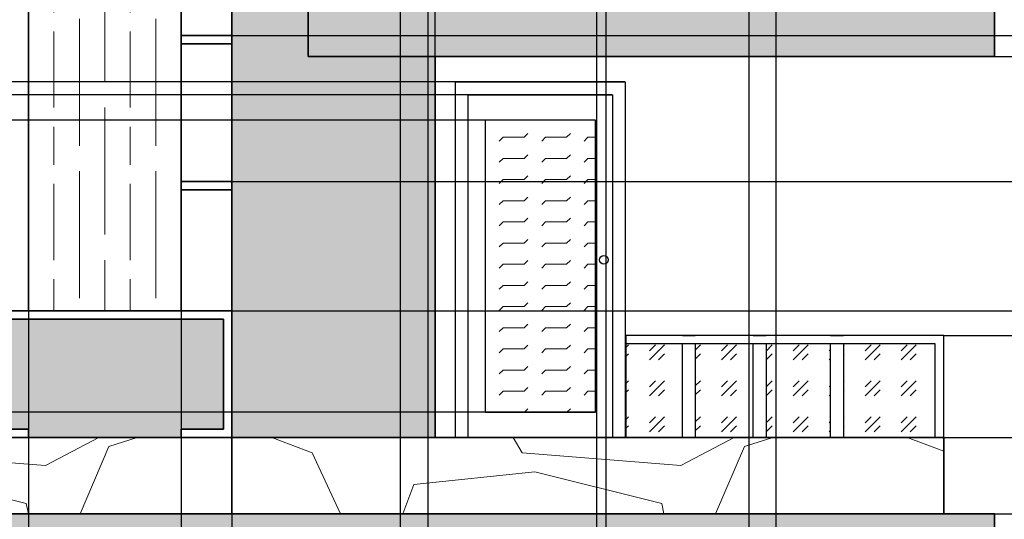
# Model space of a CAD drawing. Units: inches. Extents: x -73 to 458, y -161 to 332.
# Tile 3 of 6: x 106 to 338, y 5 to 123. Entities that reach past the tile are written whole.
import ezdxf

# ---------------------------------------------------------------- set-up
doc = ezdxf.new("R2010")
doc.units = ezdxf.units.IN
doc.header["$MEASUREMENT"] = 0
for name, color, linetype, lineweight in [('A-ANNO-DIMS', 2, 'Continuous', 18), ('A-DOOR', 4, 'Continuous', 25), ('A-ELEV', 7, 'Continuous', 35), ('A-ELEV-PATT', 8, 'Continuous', 13), ('A-GLAZ', 3, 'Continuous', 25), ('A-GLAZ-PATT', 8, 'Continuous', 13)]:
    doc.layers.add(name, color=color, linetype=linetype, lineweight=lineweight)
doc.styles.get("Standard").update_dxf_attribs({"font": 'arial.ttf'})
doc.dimstyles.get("Standard").update_dxf_attribs({"dimtxt": 12, "dimasz": 0.18, "dimexe": 0.18, "dimexo": 0.0625, "dimgap": 0.09, "dimtad": 0, "dimtih": 1, "dimtoh": 1, "dimdec": 0, "dimzin": 0, "dimdsep": 46, "dimlunit": 3, "dimtxsty": 'Standard', "dimcen": 0.09, "dimadec": 0, "dimazin": 0, "dimtfac": 1, "dimtdec": 0, "dimtofl": 0, "dimtmove": 0, "dimatfit": 3, "dimfxl": 1, "dimtolj": 1, "dimtzin": 0, "dimarcsym": 0})

# ---------------------------------------------------------------- blocks, each defined once
blk = doc.blocks.new('*U3')
blk.add_lwpolyline([(3.12, 0.01), (0.12, 0.01), (0.12, 84.01), (40.12, 84.01), (40.12, 0.01), (37.12, 0.01)])
for points in [[(37.12, 80.99), (37.12, 0.01), (3.12, 0.01), (3.12, 80.99)], [(33.12, 6.01), (33.12, 74.99), (7.12, 74.99), (7.12, 6.01)]]:
    blk.add_lwpolyline(points, close=True)
blk.add_circle((35.12, 42.01), 1)
blk = doc.blocks.new('*D7')
at = {"layer": 'A-ANNO-DIMS', "color": 0, "lineweight": -2, "transparency": 16777216}
for p, q in [((174, 126.13), (174, 324.4)), ((174.18, 324.22), (180.34, 324.22)), ((203.82, 324.22), (197.66, 324.22)), ((204, 24.13), (204, 324.4))]:
    blk.add_line(p, q, dxfattribs=at)
at = {"layer": 'A-ANNO-DIMS', "color": 0, "transparency": 16777216}
for points in [[(174.18, 324.25), (174.18, 324.19), (174, 324.22)], [(203.82, 324.25), (203.82, 324.19), (204, 324.22)]]:
    blk.add_solid(points, dxfattribs=at)
at = {"layer": 'Defpoints', "color": 0, "transparency": 16777216}
for p in [(204, 324.22), (174, 126.07), (204, 24.07)]:
    blk.add_point(p, dxfattribs=at)
at = {"layer": 'A-ANNO-DIMS', "color": 0, "transparency": 16777216, "insert": (189, 324.22), "char_height": 12, "attachment_point": 5}
blk.add_mtext('\\A1;30', dxfattribs=at)
blk = doc.blocks.new('*D8')
at = {"layer": 'A-ANNO-DIMS', "color": 0, "lineweight": -2, "transparency": 16777216}
for p, q in [((204, 24.13), (204, 324.4)), ((204.18, 324.22), (257.28, 324.22)), ((335.82, 324.22), (282.72, 324.22)), ((336, 126.13), (336, 324.4))]:
    blk.add_line(p, q, dxfattribs=at)
at = {"layer": 'A-ANNO-DIMS', "color": 0, "transparency": 16777216}
for points in [[(204.18, 324.25), (204.18, 324.19), (204, 324.22)], [(335.82, 324.25), (335.82, 324.19), (336, 324.22)]]:
    blk.add_solid(points, dxfattribs=at)
at = {"layer": 'Defpoints', "color": 0, "transparency": 16777216}
for p in [(336, 324.22), (336, 126.07), (204, 24.07)]:
    blk.add_point(p, dxfattribs=at)
at = {"layer": 'A-ANNO-DIMS', "color": 0, "transparency": 16777216, "insert": (270, 324.22), "char_height": 12, "attachment_point": 5}
blk.add_mtext('\\A1;132', dxfattribs=at)
blk = doc.blocks.new('*D18')
at = {"layer": 'A-ANNO-DIMS', "color": 0, "lineweight": -2, "transparency": 16777216}
for p, q in [((336.06, 6.07), (408.51, 6.07)), ((408.33, 6.07), (408.33, 6.25)), ((408.33, 6.25), (408.51, 6.25)), ((408.33, -5.75), (408.33, 5.89)), ((336.06, -5.93), (408.51, -5.93))]:
    blk.add_line(p, q, dxfattribs=at)
at = {"layer": 'A-ANNO-DIMS', "color": 0, "transparency": 16777216}
for points in [[(408.3, 5.89), (408.36, 5.89), (408.33, 6.07)], [(408.3, -5.75), (408.36, -5.75), (408.33, -5.93)]]:
    blk.add_solid(points, dxfattribs=at)
at = {"layer": 'Defpoints', "color": 0, "transparency": 16777216}
for p in [(336, 6.07), (408.33, 6.07), (336, -5.93)]:
    blk.add_point(p, dxfattribs=at)
at = {"layer": 'A-ANNO-DIMS', "color": 0, "transparency": 16777216, "insert": (416.56, 6.25), "char_height": 12, "attachment_point": 5}
blk.add_mtext('\\A1;12', dxfattribs=at)
blk = doc.blocks.new('*D20')
at = {"layer": 'A-ANNO-DIMS', "color": 0, "lineweight": -2, "transparency": 16777216}
for p, q in [((336.06, 114.07), (408.51, 114.07)), ((408.33, 113.89), (408.33, 66.28)), ((408.33, 6.25), (408.33, 53.85)), ((324.06, 6.07), (408.51, 6.07))]:
    blk.add_line(p, q, dxfattribs=at)
at = {"layer": 'A-ANNO-DIMS', "color": 0, "transparency": 16777216}
for points in [[(408.3, 113.89), (408.36, 113.89), (408.33, 114.07)], [(408.3, 6.25), (408.36, 6.25), (408.33, 6.07)]]:
    blk.add_solid(points, dxfattribs=at)
at = {"layer": 'Defpoints', "color": 0, "transparency": 16777216}
for p in [(336, 114.07), (408.33, 114.07), (324, 6.07)]:
    blk.add_point(p, dxfattribs=at)
at = {"layer": 'A-ANNO-DIMS', "color": 0, "transparency": 16777216, "insert": (408.33, 60.07), "char_height": 12, "attachment_point": 5}
blk.add_mtext('\\A1;108', dxfattribs=at)
blk = doc.blocks.new('*D21')
at = {"layer": 'A-ANNO-DIMS', "color": 0, "lineweight": -2, "transparency": 16777216}
for p, q in [((336.06, 126.07), (408.51, 126.07)), ((408.33, 126.07), (408.33, 126.25)), ((408.33, 126.25), (408.51, 126.25)), ((408.33, 114.25), (408.33, 125.89)), ((336.06, 114.07), (408.51, 114.07))]:
    blk.add_line(p, q, dxfattribs=at)
at = {"layer": 'A-ANNO-DIMS', "color": 0, "transparency": 16777216}
for points in [[(408.3, 125.89), (408.36, 125.89), (408.33, 126.07)], [(408.3, 114.25), (408.36, 114.25), (408.33, 114.07)]]:
    blk.add_solid(points, dxfattribs=at)
at = {"layer": 'Defpoints', "color": 0, "transparency": 16777216}
for p in [(336, 126.07), (408.33, 126.07), (336, 114.07)]:
    blk.add_point(p, dxfattribs=at)
at = {"layer": 'A-ANNO-DIMS', "color": 0, "transparency": 16777216, "insert": (416.56, 126.25), "char_height": 12, "attachment_point": 5}
blk.add_mtext('\\A1;12', dxfattribs=at)
blk = doc.blocks.new('*D36')
at = {"layer": 'A-ANNO-DIMS', "color": 0, "lineweight": -2, "transparency": 16777216}
for p, q in [((96, 53.96), (96, -153.17)), ((108, 53.96), (108, -153.17)), ((96.18, -152.99), (107.82, -152.99)), ((108, -152.99), (108.18, -152.99))]:
    blk.add_line(p, q, dxfattribs=at)
at = {"layer": 'A-ANNO-DIMS', "color": 0, "transparency": 16777216}
for points in [[(96.18, -152.96), (96.18, -153.02), (96, -152.99)], [(107.82, -152.96), (107.82, -153.02), (108, -152.99)]]:
    blk.add_solid(points, dxfattribs=at)
at = {"layer": 'Defpoints', "color": 0, "transparency": 16777216}
for p in [(96, 54.03), (108, 54.03), (108, -152.99)]:
    blk.add_point(p, dxfattribs=at)
at = {"layer": 'A-ANNO-DIMS', "color": 0, "transparency": 16777216, "insert": (116.24, -152.99), "char_height": 12, "attachment_point": 5}
blk.add_mtext('\\A1;12', dxfattribs=at)
blk = doc.blocks.new('*D37')
at = {"layer": 'A-ANNO-DIMS', "color": 0, "lineweight": -2, "transparency": 16777216}
for p, q in [((108, 53.96), (108, -153.17)), ((144, 53.96), (144, -153.17)), ((108.18, -152.99), (117.32, -152.99)), ((143.82, -152.99), (134.67, -152.99))]:
    blk.add_line(p, q, dxfattribs=at)
at = {"layer": 'A-ANNO-DIMS', "color": 0, "transparency": 16777216}
for points in [[(108.18, -152.96), (108.18, -153.02), (108, -152.99)], [(143.82, -152.96), (143.82, -153.02), (144, -152.99)]]:
    blk.add_solid(points, dxfattribs=at)
at = {"layer": 'Defpoints', "color": 0, "transparency": 16777216}
for p in [(108, 54.03), (144, 54.03), (144, -152.99)]:
    blk.add_point(p, dxfattribs=at)
at = {"layer": 'A-ANNO-DIMS', "color": 0, "transparency": 16777216, "insert": (126, -152.99), "char_height": 12, "attachment_point": 5}
blk.add_mtext('\\A1;36', dxfattribs=at)
blk = doc.blocks.new('*D38')
at = {"layer": 'A-ANNO-DIMS', "color": 0, "lineweight": -2, "transparency": 16777216}
for p, q in [((144, 53.96), (144, -153.17)), ((156, 53.96), (156, -153.17)), ((144.18, -152.99), (155.82, -152.99)), ((156, -152.99), (156.18, -152.99))]:
    blk.add_line(p, q, dxfattribs=at)
at = {"layer": 'A-ANNO-DIMS', "color": 0, "transparency": 16777216}
for points in [[(144.18, -152.96), (144.18, -153.02), (144, -152.99)], [(155.82, -152.96), (155.82, -153.02), (156, -152.99)]]:
    blk.add_solid(points, dxfattribs=at)
at = {"layer": 'Defpoints', "color": 0, "transparency": 16777216}
for p in [(144, 54.03), (156, 54.03), (156, -152.99)]:
    blk.add_point(p, dxfattribs=at)
at = {"layer": 'A-ANNO-DIMS', "color": 0, "transparency": 16777216, "insert": (164.24, -152.99), "char_height": 12, "attachment_point": 5}
blk.add_mtext('\\A1;12', dxfattribs=at)
blk = doc.blocks.new('*D39')
at = {"layer": 'A-ANNO-DIMS', "color": 0, "lineweight": -2, "transparency": 16777216}
for p, q in [((144.06, 54.03), (408.51, 54.03)), ((408.33, 53.85), (408.33, 45.26)), ((408.33, 24.25), (408.33, 32.83)), ((144.06, 24.07), (408.51, 24.07))]:
    blk.add_line(p, q, dxfattribs=at)
at = {"layer": 'A-ANNO-DIMS', "color": 0, "transparency": 16777216}
for points in [[(408.3, 53.85), (408.36, 53.85), (408.33, 54.03)], [(408.3, 24.25), (408.36, 24.25), (408.33, 24.07)]]:
    blk.add_solid(points, dxfattribs=at)
at = {"layer": 'Defpoints', "color": 0, "transparency": 16777216}
for p in [(144, 54.03), (408.33, 54.03), (144, 24.07)]:
    blk.add_point(p, dxfattribs=at)
at = {"layer": 'A-ANNO-DIMS', "color": 0, "transparency": 16777216, "insert": (408.33, 39.05), "char_height": 12, "attachment_point": 5}
blk.add_mtext('\\A1;29.96', dxfattribs=at)
blk = doc.blocks.new('*D40')
at = {"layer": 'A-ANNO-DIMS', "color": 0, "lineweight": -2, "transparency": 16777216}
for p, q in [((144.06, 84.57), (408.51, 84.57)), ((408.33, 84.39), (408.33, 75.52)), ((408.33, 54.21), (408.33, 63.08)), ((144.06, 54.03), (408.51, 54.03))]:
    blk.add_line(p, q, dxfattribs=at)
at = {"layer": 'A-ANNO-DIMS', "color": 0, "transparency": 16777216}
for points in [[(408.3, 84.39), (408.36, 84.39), (408.33, 84.57)], [(408.3, 54.21), (408.36, 54.21), (408.33, 54.03)]]:
    blk.add_solid(points, dxfattribs=at)
at = {"layer": 'Defpoints', "color": 0, "transparency": 16777216}
for p in [(144, 84.57), (408.33, 84.57), (144, 54.03)]:
    blk.add_point(p, dxfattribs=at)
at = {"layer": 'A-ANNO-DIMS', "color": 0, "transparency": 16777216, "insert": (408.33, 69.3), "char_height": 12, "attachment_point": 5}
blk.add_mtext('\\A1;30.546', dxfattribs=at)
blk = doc.blocks.new('*D41')
at = {"layer": 'A-ANNO-DIMS', "color": 0, "lineweight": -2, "transparency": 16777216}
for p, q in [((144.06, 119.06), (408.51, 119.06)), ((408.33, 118.88), (408.33, 108.04)), ((408.33, 84.75), (408.33, 95.59)), ((144.06, 84.57), (408.51, 84.57))]:
    blk.add_line(p, q, dxfattribs=at)
at = {"layer": 'A-ANNO-DIMS', "color": 0, "transparency": 16777216}
for points in [[(408.3, 118.88), (408.36, 118.88), (408.33, 119.06)], [(408.3, 84.75), (408.36, 84.75), (408.33, 84.57)]]:
    blk.add_solid(points, dxfattribs=at)
at = {"layer": 'Defpoints', "color": 0, "transparency": 16777216}
for p in [(144, 119.06), (408.33, 119.06), (144, 84.57)]:
    blk.add_point(p, dxfattribs=at)
at = {"layer": 'A-ANNO-DIMS', "color": 0, "transparency": 16777216, "insert": (408.33, 101.81), "char_height": 12, "attachment_point": 5}
blk.add_mtext('\\A1;34.484', dxfattribs=at)
blk = doc.blocks.new('*D42')
at = {"layer": 'A-ANNO-DIMS', "color": 0, "lineweight": -2, "transparency": 16777216}
for p, q in [((144.06, 149.14), (408.51, 149.14)), ((408.33, 148.96), (408.33, 140.32)), ((408.33, 119.24), (408.33, 127.88)), ((144.06, 119.06), (408.51, 119.06))]:
    blk.add_line(p, q, dxfattribs=at)
at = {"layer": 'A-ANNO-DIMS', "color": 0, "transparency": 16777216}
for points in [[(408.3, 148.96), (408.36, 148.96), (408.33, 149.14)], [(408.3, 119.24), (408.36, 119.24), (408.33, 119.06)]]:
    blk.add_solid(points, dxfattribs=at)
at = {"layer": 'Defpoints', "color": 0, "transparency": 16777216}
for p in [(144, 149.14), (408.33, 149.14), (144, 119.06)]:
    blk.add_point(p, dxfattribs=at)
at = {"layer": 'A-ANNO-DIMS', "color": 0, "transparency": 16777216, "insert": (408.33, 134.1), "char_height": 12, "attachment_point": 5}
blk.add_mtext('\\A1;30.08', dxfattribs=at)
blk = doc.blocks.new('*D65')
at = {"layer": 'A-ANNO-DIMS', "color": 0, "lineweight": -2, "transparency": 16777216}
for p, q in [((-41.6, 30.08), (-41.6, 30.26)), ((-41.6, 30.26), (-41.42, 30.26)), ((241.74, 30.08), (-41.78, 30.08)), ((-41.6, 24.26), (-41.6, 29.9)), ((248.74, 24.08), (-41.78, 24.08))]:
    blk.add_line(p, q, dxfattribs=at)
at = {"layer": 'A-ANNO-DIMS', "color": 0, "transparency": 16777216}
for points in [[(-41.63, 29.9), (-41.57, 29.9), (-41.6, 30.08)], [(-41.63, 24.26), (-41.57, 24.26), (-41.6, 24.08)]]:
    blk.add_solid(points, dxfattribs=at)
at = {"layer": 'Defpoints', "color": 0, "transparency": 16777216}
for p in [(-41.6, 30.08), (241.81, 30.08), (248.81, 24.08)]:
    blk.add_point(p, dxfattribs=at)
at = {"layer": 'A-ANNO-DIMS', "color": 0, "transparency": 16777216, "insert": (-37.37, 30.26), "char_height": 12, "attachment_point": 5}
blk.add_mtext('\\A1;6', dxfattribs=at)
blk = doc.blocks.new('*D66')
at = {"layer": 'A-ANNO-DIMS', "color": 0, "lineweight": -2, "transparency": 16777216}
for p, q in [((241.74, 99.06), (-41.78, 99.06)), ((-41.6, 98.88), (-41.6, 70.78)), ((-41.6, 30.26), (-41.6, 58.35)), ((241.74, 30.08), (-41.78, 30.08))]:
    blk.add_line(p, q, dxfattribs=at)
at = {"layer": 'A-ANNO-DIMS', "color": 0, "transparency": 16777216}
for points in [[(-41.63, 98.88), (-41.57, 98.88), (-41.6, 99.06)], [(-41.63, 30.26), (-41.57, 30.26), (-41.6, 30.08)]]:
    blk.add_solid(points, dxfattribs=at)
at = {"layer": 'Defpoints', "color": 0, "transparency": 16777216}
for p in [(-41.6, 99.06), (241.81, 99.06), (241.81, 30.08)]:
    blk.add_point(p, dxfattribs=at)
at = {"layer": 'A-ANNO-DIMS', "color": 0, "transparency": 16777216, "insert": (-41.6, 64.57), "char_height": 12, "attachment_point": 5}
blk.add_mtext('\\A1;68.98', dxfattribs=at)
blk = doc.blocks.new('*D67')
at = {"layer": 'A-ANNO-DIMS', "color": 0, "lineweight": -2, "transparency": 16777216}
for p, q in [((245.74, 105.06), (-41.78, 105.06)), ((-41.6, 105.06), (-41.6, 105.24)), ((-41.6, 105.24), (-41.42, 105.24)), ((-41.6, 99.24), (-41.6, 104.88)), ((241.74, 99.06), (-41.78, 99.06))]:
    blk.add_line(p, q, dxfattribs=at)
at = {"layer": 'A-ANNO-DIMS', "color": 0, "transparency": 16777216}
for points in [[(-41.63, 104.88), (-41.57, 104.88), (-41.6, 105.06)], [(-41.63, 99.24), (-41.57, 99.24), (-41.6, 99.06)]]:
    blk.add_solid(points, dxfattribs=at)
at = {"layer": 'Defpoints', "color": 0, "transparency": 16777216}
for p in [(-41.6, 105.06), (245.81, 105.06), (241.81, 99.06)]:
    blk.add_point(p, dxfattribs=at)
at = {"layer": 'A-ANNO-DIMS', "color": 0, "transparency": 16777216, "insert": (-37.37, 105.24), "char_height": 12, "attachment_point": 5}
blk.add_mtext('\\A1;6', dxfattribs=at)
blk = doc.blocks.new('*D68')
at = {"layer": 'A-ANNO-DIMS', "color": 0, "lineweight": -2, "transparency": 16777216}
for p, q in [((248.74, 108.08), (-41.78, 108.08)), ((-41.6, 108.08), (-41.6, 108.26)), ((-41.6, 108.26), (-41.42, 108.26)), ((-41.6, 105.24), (-41.6, 107.9)), ((245.74, 105.06), (-41.78, 105.06))]:
    blk.add_line(p, q, dxfattribs=at)
at = {"layer": 'A-ANNO-DIMS', "color": 0, "transparency": 16777216}
for points in [[(-41.63, 107.9), (-41.57, 107.9), (-41.6, 108.08)], [(-41.63, 105.24), (-41.57, 105.24), (-41.6, 105.06)]]:
    blk.add_solid(points, dxfattribs=at)
at = {"layer": 'Defpoints', "color": 0, "transparency": 16777216}
for p in [(-41.6, 108.08), (248.81, 108.08), (245.81, 105.06)]:
    blk.add_point(p, dxfattribs=at)
at = {"layer": 'A-ANNO-DIMS', "color": 0, "transparency": 16777216, "insert": (-21.09, 108.26), "char_height": 12, "attachment_point": 5}
blk.add_mtext('\\A1;3.023', dxfattribs=at)
blk = doc.blocks.new('*D70')
at = {"layer": 'A-ANNO-DIMS', "color": 0, "lineweight": -2, "transparency": 16777216}
for p, q in [((324.06, 48.19), (408.51, 48.19)), ((408.33, 48.01), (408.33, 42.35)), ((408.33, 24.25), (408.33, 29.91)), ((324.06, 24.07), (408.51, 24.07))]:
    blk.add_line(p, q, dxfattribs=at)
at = {"layer": 'A-ANNO-DIMS', "color": 0, "transparency": 16777216}
for points in [[(408.3, 48.01), (408.36, 48.01), (408.33, 48.19)], [(408.3, 24.25), (408.36, 24.25), (408.33, 24.07)]]:
    blk.add_solid(points, dxfattribs=at)
at = {"layer": 'Defpoints', "color": 0, "transparency": 16777216}
for p in [(324, 48.19), (408.33, 48.19), (324, 24.07)]:
    blk.add_point(p, dxfattribs=at)
at = {"layer": 'A-ANNO-DIMS', "color": 0, "transparency": 16777216, "insert": (408.33, 36.13), "char_height": 12, "attachment_point": 5}
blk.add_mtext('\\A1;24.125', dxfattribs=at)
blk = doc.blocks.new('*D71')
at = {"layer": 'A-ANNO-DIMS', "color": 0, "lineweight": -2, "transparency": 16777216}
for p, q in [((195.77, -5.87), (195.77, 324.4)), ((195.95, 324.22), (202.17, 324.22)), ((202.35, -5.87), (202.35, 324.4)), ((202.35, 324.22), (202.53, 324.22))]:
    blk.add_line(p, q, dxfattribs=at)
at = {"layer": 'A-ANNO-DIMS', "color": 0, "transparency": 16777216}
for points in [[(195.95, 324.25), (195.95, 324.19), (195.77, 324.22)], [(202.17, 324.25), (202.17, 324.19), (202.35, 324.22)]]:
    blk.add_solid(points, dxfattribs=at)
at = {"layer": 'Defpoints', "color": 0, "transparency": 16777216}
for p in [(202.35, 324.22), (195.77, -5.93), (202.35, -5.93)]:
    blk.add_point(p, dxfattribs=at)
at = {"layer": 'A-ANNO-DIMS', "color": 0, "transparency": 16777216, "insert": (222.95, 324.22), "char_height": 12, "attachment_point": 5}
blk.add_mtext('\\A1;6.585', dxfattribs=at)
blk = doc.blocks.new('*D72')
at = {"layer": 'A-ANNO-DIMS', "color": 0, "lineweight": -2, "transparency": 16777216}
for p, q in [((202.35, -5.87), (202.35, 324.4)), ((202.53, 324.22), (241.93, 324.22)), ((242.11, -5.87), (242.11, 324.4)), ((242.11, 324.22), (242.29, 324.22))]:
    blk.add_line(p, q, dxfattribs=at)
at = {"layer": 'A-ANNO-DIMS', "color": 0, "transparency": 16777216}
for points in [[(202.53, 324.25), (202.53, 324.19), (202.35, 324.22)], [(241.93, 324.25), (241.93, 324.19), (242.11, 324.22)]]:
    blk.add_solid(points, dxfattribs=at)
at = {"layer": 'Defpoints', "color": 0, "transparency": 16777216}
for p in [(242.11, 324.22), (202.35, -5.93), (242.11, -5.93)]:
    blk.add_point(p, dxfattribs=at)
at = {"layer": 'A-ANNO-DIMS', "color": 0, "transparency": 16777216, "insert": (262.62, 324.22), "char_height": 12, "attachment_point": 5}
blk.add_mtext('\\A1;39.76', dxfattribs=at)
blk = doc.blocks.new('*D73')
at = {"layer": 'A-ANNO-DIMS', "color": 0, "lineweight": -2, "transparency": 16777216}
for p, q in [((242.11, -5.87), (242.11, 324.4)), ((242.29, 324.22), (244.17, 324.22)), ((244.35, -5.87), (244.35, 324.4)), ((244.35, 324.22), (244.53, 324.22))]:
    blk.add_line(p, q, dxfattribs=at)
at = {"layer": 'A-ANNO-DIMS', "color": 0, "transparency": 16777216}
for points in [[(242.29, 324.25), (242.29, 324.19), (242.11, 324.22)], [(244.17, 324.25), (244.17, 324.19), (244.35, 324.22)]]:
    blk.add_solid(points, dxfattribs=at)
at = {"layer": 'Defpoints', "color": 0, "transparency": 16777216}
for p in [(244.35, 324.22), (242.11, -5.93), (244.35, -5.93)]:
    blk.add_point(p, dxfattribs=at)
at = {"layer": 'A-ANNO-DIMS', "color": 0, "transparency": 16777216, "insert": (264.95, 324.22), "char_height": 12, "attachment_point": 5}
blk.add_mtext('\\A1;2.244', dxfattribs=at)
blk = doc.blocks.new('*D74')
at = {"layer": 'A-ANNO-DIMS', "color": 0, "lineweight": -2, "transparency": 16777216}
for p, q in [((244.35, -5.87), (244.35, 324.4)), ((244.53, 324.22), (277.93, 324.22)), ((278.11, -5.87), (278.11, 324.4)), ((278.11, 324.22), (278.29, 324.22))]:
    blk.add_line(p, q, dxfattribs=at)
at = {"layer": 'A-ANNO-DIMS', "color": 0, "transparency": 16777216}
for points in [[(244.53, 324.25), (244.53, 324.19), (244.35, 324.22)], [(277.93, 324.25), (277.93, 324.19), (278.11, 324.22)]]:
    blk.add_solid(points, dxfattribs=at)
at = {"layer": 'Defpoints', "color": 0, "transparency": 16777216}
for p in [(278.11, 324.22), (244.35, -5.93), (278.11, -5.93)]:
    blk.add_point(p, dxfattribs=at)
at = {"layer": 'A-ANNO-DIMS', "color": 0, "transparency": 16777216, "insert": (303.28, 324.22), "char_height": 12, "attachment_point": 5}
blk.add_mtext('\\A1;33.756', dxfattribs=at)
blk = doc.blocks.new('*D75')
at = {"layer": 'A-ANNO-DIMS', "color": 0, "lineweight": -2, "transparency": 16777216}
for p, q in [((278.11, -5.87), (278.11, 324.4)), ((278.29, 324.22), (284.3, 324.22)), ((284.48, -5.87), (284.48, 324.4)), ((284.48, 324.22), (284.66, 324.22))]:
    blk.add_line(p, q, dxfattribs=at)
at = {"layer": 'A-ANNO-DIMS', "color": 0, "transparency": 16777216}
for points in [[(278.29, 324.25), (278.29, 324.19), (278.11, 324.22)], [(284.3, 324.25), (284.3, 324.19), (284.48, 324.22)]]:
    blk.add_solid(points, dxfattribs=at)
at = {"layer": 'Defpoints', "color": 0, "transparency": 16777216}
for p in [(284.48, 324.22), (278.11, -5.93), (284.48, -5.93)]:
    blk.add_point(p, dxfattribs=at)
at = {"layer": 'A-ANNO-DIMS', "color": 0, "transparency": 16777216, "insert": (305.03, 324.22), "char_height": 12, "attachment_point": 5}
blk.add_mtext('\\A1;6.377', dxfattribs=at)

msp = doc.modelspace()

# ---------------------------------------------------------------- hatches: boundary and pattern name
at = {"layer": 'A-ELEV-PATT'}
h = msp.add_hatch(color=256, dxfattribs=at)
h.dxf.hatch_style = 1
h.paths.add_polyline_path([(167.9979, 302.0202), (155.9979, 302.0202), (95.9979, 302.0202), (23.9979, 302.0202), (23.9979, -113.9335), (33.9979, -113.9335), (33.9979, 292.0202), (95.9979, 292.0202), (157.9979, 292.0202), (157.9979, 260.2059), (167.9979, 260.2059), (167.9979, 290.0202)])
h.paths.add_polyline_path([(335.9979, 242.2059), (323.9979, 242.2059), (95.9979, 242.2059), (95.9979, 234.0665), (95.9979, 230.2059), (323.9979, 230.2059), (335.9979, 230.2059)])
h.paths.add_polyline_path([(335.9979, 126.0665), (323.9979, 126.0665), (173.9979, 126.0665), (173.9979, 114.0665), (323.9979, 114.0665), (335.9979, 114.0665)])
h.paths.add_polyline_path([(335.9979, 6.0665), (323.9979, 6.0665), (95.9979, 6.0665), (95.9979, -5.9335), (323.9979, -5.9335), (335.9979, -5.9335)])
h = msp.add_hatch(dxfattribs=at)
h.set_pattern_fill('GRAVEL', color=256, scale=150)
h.paths.add_polyline_path([(95.9979, 234.0665), (95.9979, 260.2059), (155.9979, 260.2059), (155.9979, 290.0202), (95.9979, 290.0202), (55.9979, 290.0202), (55.9979, -113.9335), (95.9979, -113.9335), (95.9979, 24.0665), (95.9979, 54.0267)])
h.paths.add_polyline_path([(323.9979, 144.0665), (248.9979, 144.0665), (173.9979, 144.0665), (173.9979, 126.0665), (323.9979, 126.0665)])
h.paths.add_polyline_path([(323.9979, 24.0665), (248.9979, 24.0665), (155.9979, 24.0665), (155.9979, 6.0665), (323.9979, 6.0665)])
h.paths.add_polyline_path([(323.9979, 260.2059), (95.9979, 260.2059), (95.9979, 242.2059), (323.9979, 242.2059)])
h.paths.add_polyline_path([(155.9979, 24.0665), (95.9979, 24.0665), (95.9979, 6.0665), (155.9979, 6.0665)], flags=17)
h = msp.add_hatch(color=256, dxfattribs=at)
h.dxf.hatch_style = 1
h.paths.add_polyline_path([(195.7666, -5.9335), (155.3839, -5.9335), (155.3839, -113.9335), (195.7666, -113.9335)])
h.paths.add_polyline_path([(323.9979, -5.9335), (284.4845, -5.9335), (284.4845, -113.9335), (323.9979, -113.9335)])
h.paths.add_polyline_path([(203.9979, 114.0665), (173.9979, 114.0665), (173.9979, 144.0665), (203.9979, 144.0665), (203.9979, 230.2059), (155.9979, 230.2059), (155.9979, 24.0665), (203.9979, 24.0665)])
h = msp.add_hatch(dxfattribs=at)
h.set_pattern_fill('FLEX', color=256, scale=20)
h.paths.add_polyline_path([(241.805, 219.0563), (215.805, 219.0563), (215.805, 150.0793), (241.805, 150.0793)])
h.paths.add_polyline_path([(241.805, 99.0563), (215.805, 99.0563), (215.805, 30.0793), (241.805, 30.0793)])
h.paths.add_polyline_path([(138.915, -38.9437), (112.915, -38.9437), (112.915, -107.9207), (138.915, -107.9207)])
h = msp.add_hatch(dxfattribs=at)
h.set_pattern_fill('GOST_WOOD', color=256, scale=3)
h.set_pattern_definition([(90, (0, 0), (18, -1e-15), [30, -6]), (90, (6, -6), (18, -1e-15), [18, -4.5, 9, -4.5]), (90, (12, -15), (18, -1e-15), [30, -6])])
h.paths.add_polyline_path([(143.9979, 215.8003), (107.9979, 215.8003), (107.9979, 54.0267), (143.9979, 54.0267)])
h = msp.add_hatch(color=256, dxfattribs=at)
h.dxf.hatch_style = 1
h.paths.add_polyline_path([(153.9979, 52.0267), (97.9979, 52.0267), (97.9979, 26.0665), (107.9979, 26.0665), (107.9979, 24.0665), (143.9979, 24.0665), (143.9979, 26.0665), (153.9979, 26.0665)])

# ---------------------------------------------------------------- linework, layer by layer
at = {"layer": 'A-ELEV'}
for p, q in [((155.9979, 6.0665), (155.9979, 230.2059)), ((107.9979, 215.8003), (107.9979, 54.0267)), ((143.9979, 54.0267), (143.9979, 215.8003)), ((173.9979, 144.0665), (173.9979, 114.0665)), ((323.9979, 114.0665), (173.9979, 114.0665)), ((203.9979, 24.0665), (203.9979, 114.0665)), ((107.9979, 26.0665), (107.9979, 24.0665)), ((143.9979, 24.0665), (143.9979, 26.0665)), ((95.9979, 24.0665), (143.9979, 24.0665)), ((155.9979, 24.0665), (323.9979, 24.0665)), ((323.9979, 6.0665), (323.9979, 24.0665)), ((95.9979, 6.0665), (323.9979, 6.0665))]:
    msp.add_line(p, q, dxfattribs=at)
for points in [[(323.9979, 126.0665), (335.9979, 126.0665), (335.9979, 114.0665), (323.9979, 114.0665)], [(155.9979, 56.0043), (155.9979, 54.0267), (143.9979, 54.0267), (143.9979, 56.0043)], [(143.9979, 26.0665), (153.9979, 26.0665), (153.9979, 52.0267), (97.9979, 52.0267), (97.9979, 26.0665), (107.9979, 26.0665)], [(143.9979, 24.6791), (143.9979, 25.9247)], [(155.9979, 25.9247), (155.9979, 24.6791)], [(323.9979, 6.0665), (335.9979, 6.0665), (335.9979, -5.9335), (323.9979, -5.9335)]]:
    msp.add_lwpolyline(points, dxfattribs=at)
for points in [[(143.9979, 119.0564), (155.9979, 119.0564), (155.9979, 117.0789), (143.9979, 117.0789)], [(143.9979, 84.5727), (155.9979, 84.5727), (155.9979, 82.5952), (143.9979, 82.5952)], [(95.9979, 24.0665), (155.9979, 24.0665), (155.9979, 54.0267), (95.9979, 54.0267)]]:
    msp.add_lwpolyline(points, close=True, dxfattribs=at)
at = {"layer": 'A-GLAZ'}
for p, q in [((248.9979, 48.1912), (248.9979, 24.0665)), ((248.9979, 24.0665), (323.9979, 24.0665))]:
    msp.add_line(p, q, dxfattribs=at)
for points in [[(323.9979, 24.0665), (323.9979, 48.1912), (248.9979, 48.1912)], [(262.3267, 48.1912), (265.3698, 48.1912)], [(279.0639, 48.1912), (282.107, 48.1912)], [(297.3226, 48.1912), (300.3657, 48.1912)], [(321.9979, 24.0665), (321.9979, 46.1912), (248.9979, 46.1912)], [(265.3698, 46.1912), (265.3698, 24.0665), (262.3267, 24.0665), (262.3267, 46.1912)], [(282.107, 46.1912), (282.107, 24.0665), (279.0639, 24.0665), (279.0639, 46.1912)], [(300.3657, 46.1912), (300.3657, 24.0665), (297.3226, 24.0665), (297.3226, 46.1912)]]:
    msp.add_lwpolyline(points, dxfattribs=at)
at = {"layer": 'A-GLAZ-PATT'}
for p, q in [((248.9979, 45.3511), (249.6087, 45.9619)), ((254.5584, 42.4264), (258.094, 45.9619)), ((254.5584, 44.5477), (255.9727, 45.9619)), ((265.3698, 44.7525), (266.5793, 45.9619)), ((271.529, 42.4264), (275.0645, 45.9619)), ((271.529, 44.5477), (272.9432, 45.9619)), ((282.107, 44.5191), (283.5498, 45.9619)), ((288.4996, 42.4264), (292.0351, 45.9619)), ((288.4996, 44.5477), (289.9138, 45.9619)), ((296.9848, 44.5477), (297.3226, 44.8855)), ((300.3657, 45.8073), (300.5204, 45.9619)), ((305.4701, 42.4264), (309.0057, 45.9619)), ((305.4701, 44.5477), (306.8843, 45.9619)), ((313.9554, 42.4264), (317.4909, 45.9619)), ((313.9554, 44.5477), (315.3696, 45.9619)), ((248.9979, 43.2298), (249.6087, 43.8406)), ((256.6798, 42.4264), (258.094, 43.8406)), ((265.3698, 42.6312), (266.5793, 43.8406)), ((273.6503, 42.4264), (275.0645, 43.8406)), ((282.1356, 42.4264), (283.5498, 43.8406)), ((290.6209, 42.4264), (292.0351, 43.8406)), ((296.9848, 42.4264), (297.3226, 42.7642)), ((300.3657, 43.686), (300.5204, 43.8406)), ((307.5914, 42.4264), (309.0057, 43.8406)), ((316.0767, 42.4264), (317.4909, 43.8406)), ((248.9979, 36.8658), (249.6087, 37.4767)), ((254.5584, 33.9411), (258.094, 37.4767)), ((254.5584, 36.0624), (255.9727, 37.4767)), ((265.3698, 36.2672), (266.5793, 37.4767)), ((271.529, 33.9411), (275.0645, 37.4767)), ((271.529, 36.0624), (272.9432, 37.4767)), ((282.107, 36.0338), (283.5498, 37.4767)), ((288.4996, 33.9411), (292.0351, 37.4767)), ((288.4996, 36.0624), (289.9138, 37.4767)), ((300.3657, 37.322), (300.5204, 37.4767)), ((305.4701, 33.9411), (309.0057, 37.4767)), ((305.4701, 36.0624), (306.8843, 37.4767)), ((313.9554, 33.9411), (317.4909, 37.4767)), ((313.9554, 36.0624), (315.3696, 37.4767)), ((248.9979, 34.7445), (249.6087, 35.3553)), ((256.6798, 33.9411), (258.094, 35.3553)), ((265.3698, 34.1459), (266.5793, 35.3553)), ((273.6503, 33.9411), (275.0645, 35.3553)), ((282.1356, 33.9411), (283.5498, 35.3553)), ((290.6209, 33.9411), (292.0351, 35.3553)), ((296.9848, 36.0624), (297.3226, 36.4002)), ((300.3657, 35.2007), (300.5204, 35.3553)), ((307.5914, 33.9411), (309.0057, 35.3553)), ((316.0767, 33.9411), (317.4909, 35.3553)), ((296.9848, 33.9411), (297.3226, 34.2789)), ((248.9979, 28.3805), (249.6087, 28.9914)), ((254.5584, 25.4558), (258.094, 28.9914)), ((254.5584, 27.5772), (255.9727, 28.9914)), ((265.3698, 27.7819), (266.5793, 28.9914)), ((271.529, 25.4558), (275.0645, 28.9914)), ((271.529, 27.5772), (272.9432, 28.9914)), ((282.107, 27.5486), (283.5498, 28.9914)), ((288.4996, 25.4558), (292.0351, 28.9914)), ((288.4996, 27.5772), (289.9138, 28.9914)), ((296.9848, 27.5772), (297.3226, 27.9149)), ((300.3657, 28.8367), (300.5204, 28.9914)), ((305.4701, 25.4558), (309.0057, 28.9914)), ((305.4701, 27.5772), (306.8843, 28.9914)), ((313.9554, 25.4558), (317.4909, 28.9914)), ((313.9554, 27.5772), (315.3696, 28.9914)), ((248.9979, 26.2592), (249.6087, 26.8701)), ((256.6798, 25.4558), (258.094, 26.8701)), ((265.3698, 25.6606), (266.5793, 26.8701)), ((273.6503, 25.4558), (275.0645, 26.8701)), ((282.1356, 25.4558), (283.5498, 26.8701)), ((290.6209, 25.4558), (292.0351, 26.8701)), ((296.9848, 25.4558), (297.3226, 25.7936)), ((300.3657, 26.7154), (300.5204, 26.8701)), ((307.5914, 25.4558), (309.0057, 26.8701)), ((316.0767, 25.4558), (317.4909, 26.8701))]:
    msp.add_line(p, q, dxfattribs=at)

# ---------------------------------------------------------------- block references
at = {"layer": 'A-DOOR'}
msp.add_blockref('*U3', (208.6813, 24.0665), dxfattribs=at)

# ---------------------------------------------------------------- dimensions: what is measured, and where the dimension line sits
at = {"layer": 'A-ANNO-DIMS'}
for base, p1, p2, override, picture, middle in [((203.9979, 324.2202), (173.9979, 126.0665), (203.9979, 24.0665), {"dimdec": 0, "dimlfac": 1, "dimrnd": 0, "dimzin": 0, "dimdsep": 46, "dimlunit": 2}, '*D7', (188.9979, 324.2202)), ((202.3513, 324.2202), (195.7666, -5.9335), (202.3513, -5.9335), {"dimdec": 3, "dimlfac": 1, "dimrnd": 0, "dimzin": 0, "dimdsep": 46, "dimlunit": 2}, '*D71', (222.946, 324.2202)), ((242.1074, 324.2202), (202.3513, -5.9335), (242.1074, -5.9335), {"dimdec": 2, "dimlfac": 1, "dimrnd": 0, "dimzin": 0, "dimdsep": 46, "dimlunit": 2}, '*D72', (262.6161, 324.2202)), ((335.9979, 324.2202), (203.9979, 24.0665), (335.9979, 126.0665), {"dimdec": 0, "dimlfac": 1, "dimrnd": 0, "dimzin": 0, "dimdsep": 46, "dimlunit": 2}, '*D8', (269.9979, 324.2202)), ((244.3513, 324.2202), (242.1074, -5.9335), (244.3513, -5.9335), {"dimdec": 3, "dimlfac": 1, "dimrnd": 0, "dimzin": 0, "dimdsep": 46, "dimlunit": 2}, '*D73', (264.946, 324.2202)), ((278.1074, 324.2202), (244.3513, -5.9335), (278.1074, -5.9335), {"dimdec": 3, "dimlfac": 1, "dimrnd": 0, "dimzin": 0, "dimdsep": 46, "dimlunit": 2}, '*D74', (303.2778, 324.2202)), ((284.4845, 324.2202), (278.1074, -5.9335), (284.4845, -5.9335), {"dimdec": 3, "dimlfac": 1, "dimrnd": 0, "dimzin": 0, "dimdsep": 46, "dimlunit": 2}, '*D75', (305.0342, 324.2202)), ((107.9979, -152.9857), (95.9979, 54.0267), (107.9979, 54.0267), {"dimdec": 0, "dimlfac": 1, "dimrnd": 0, "dimzin": 0, "dimdsep": 46, "dimlunit": 2}, '*D36', (116.2365, -152.9857)), ((143.9979, -152.9857), (107.9979, 54.0267), (143.9979, 54.0267), {"dimdec": 0, "dimlfac": 1, "dimrnd": 0, "dimzin": 0, "dimdsep": 46, "dimlunit": 2}, '*D37', (125.9979, -152.9857)), ((155.9979, -152.9857), (143.9979, 54.0267), (155.9979, 54.0267), {"dimdec": 0, "dimlfac": 1, "dimrnd": 0, "dimzin": 0, "dimdsep": 46, "dimlunit": 2}, '*D38', (164.2365, -152.9857))]:
    dim = msp.add_linear_dim(base=base, p1=p1, p2=p2, dimstyle='Standard', override=override, dxfattribs=at)
    dim.commit()
    dim.dimension.update_dxf_attribs({"geometry": picture, "text_midpoint": middle})
for base, p1, p2, override, picture, middle in [((408.326, 149.136), (143.9979, 119.0564), (143.9979, 149.136), {"dimdec": 2, "dimlfac": 1, "dimrnd": 0, "dimzin": 0, "dimdsep": 46, "dimlunit": 2}, '*D42', (408.326, 134.0962)), ((408.326, 126.0665), (335.9979, 114.0665), (335.9979, 126.0665), {"dimdec": 0, "dimlfac": 1, "dimrnd": 0, "dimzin": 0, "dimdsep": 46, "dimlunit": 2}, '*D21', (416.5646, 126.2465)), ((408.326, 119.0564), (143.9979, 84.5727), (143.9979, 119.0564), {"dimdec": 3, "dimlfac": 1, "dimrnd": 0, "dimzin": 0, "dimdsep": 46, "dimlunit": 2}, '*D41', (408.326, 101.8146)), ((-41.6031, 108.0793), (245.805, 105.0563), (248.805, 108.0793), {"dimdec": 3, "dimlfac": 1, "dimrnd": 0, "dimzin": 0, "dimdsep": 46, "dimlunit": 2}, '*D68', (-21.0903, 108.2593)), ((408.326, 114.0665), (323.9979, 6.0665), (335.9979, 114.0665), {"dimdec": 0, "dimlfac": 1, "dimrnd": 0, "dimzin": 0, "dimdsep": 46, "dimlunit": 2}, '*D20', (408.326, 60.0665)), ((-41.6031, 105.0563), (241.805, 99.0563), (245.805, 105.0563), {"dimdec": 0, "dimlfac": 1, "dimrnd": 0, "dimzin": 0, "dimdsep": 46, "dimlunit": 2}, '*D67', (-37.3713, 105.2363)), ((-41.6031, 99.0563), (241.805, 30.0793), (241.805, 99.0563), {"dimdec": 2, "dimlfac": 1, "dimrnd": 0, "dimzin": 0, "dimdsep": 46, "dimlunit": 2}, '*D66', (-41.6031, 64.5678)), ((408.326, 84.5727), (143.9979, 54.0267), (143.9979, 84.5727), {"dimdec": 3, "dimlfac": 1, "dimrnd": 0, "dimzin": 0, "dimdsep": 46, "dimlunit": 2}, '*D40', (408.326, 69.2997)), ((408.326, 54.0267), (143.9979, 24.0665), (143.9979, 54.0267), {"dimdec": 2, "dimlfac": 1, "dimrnd": 0, "dimzin": 0, "dimdsep": 46, "dimlunit": 2}, '*D39', (408.326, 39.0466)), ((408.326, 48.1912), (323.9979, 24.0665), (323.9979, 48.1912), {"dimdec": 3, "dimlfac": 1, "dimrnd": 0, "dimzin": 0, "dimdsep": 46, "dimlunit": 2}, '*D70', (408.326, 36.1288)), ((-41.6031, 30.0793), (248.805, 24.0793), (241.805, 30.0793), {"dimdec": 0, "dimlfac": 1, "dimrnd": 0, "dimzin": 0, "dimdsep": 46, "dimlunit": 2}, '*D65', (-37.3713, 30.2593)), ((408.326, 6.0665), (335.9979, -5.9335), (335.9979, 6.0665), {"dimdec": 0, "dimlfac": 1, "dimrnd": 0, "dimzin": 0, "dimdsep": 46, "dimlunit": 2}, '*D18', (416.5646, 6.2465))]:
    dim = msp.add_linear_dim(base=base, p1=p1, p2=p2, angle=90, dimstyle='Standard', override=override, dxfattribs=at)
    dim.commit()
    dim.dimension.update_dxf_attribs({"geometry": picture, "text_midpoint": middle})

doc.saveas('drawing.dxf')
